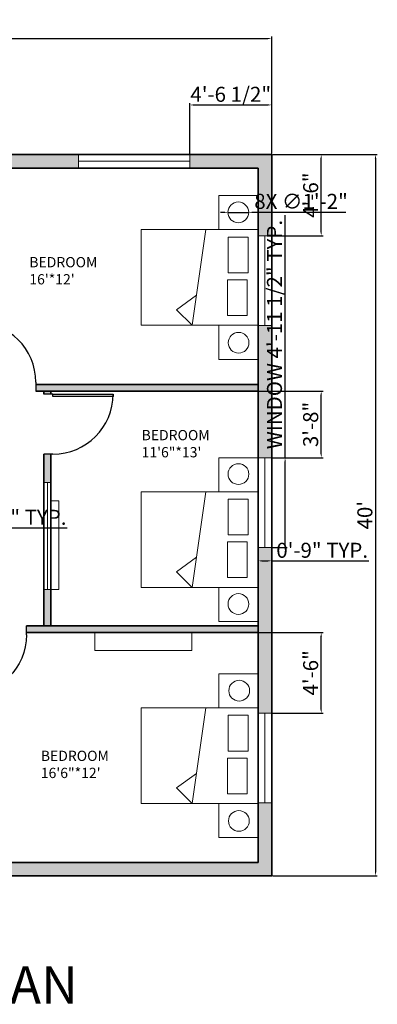
# Model space of a CAD drawing. Units: inches. Extents: x 1433 to 2137, y 2961 to 3626.
# Tile 3 of 3: x 1899 to 2137, y 2961 to 3616. Entities that reach past the tile are written whole.
import ezdxf

# ---------------------------------------------------------------- set-up
doc = ezdxf.new("R2010")
doc.units = ezdxf.units.IN
for name, color, linetype, lineweight in [('A-ANNO-DIMS', 2, 'Continuous', 18), ('A-ANNO-TEXT', 7, 'Continuous', 25), ('A-AREA-IDEN', 7, 'Continuous', 18), ('A-FURN', 8, 'Continuous', 18), ('A-WALL-PATT', 46, 'Continuous', 13), ('bed', 10, 'Continuous', 18), ('door', 50, 'Continuous', 25), ('wall', 46, 'Continuous', 35), ('window', 30, 'Continuous', 18)]:
    doc.layers.add(name, color=color, linetype=linetype, lineweight=lineweight)
doc.styles.get("Standard").update_dxf_attribs({"font": 'arial.ttf'})
doc.dimstyles.new('ISO-25', dxfattribs={"dimtxt": 10, "dimasz": 2.5, "dimexe": 1.25, "dimexo": 0.625, "dimtad": 1, "dimdec": 0, "dimlunit": 4, "dimtxsty": 'Standard', "dimcen": 2.5, "dimadec": 0, "dimazin": 0, "dimtfac": 1, "dimtdec": 0, "dimtmove": 0, "dimatfit": 3, "dimfxl": 1, "dimarcsym": 0})

# ---------------------------------------------------------------- blocks, each defined once
blk = doc.blocks.new('*U2')
for p, q in [((0, 0), (0, -6)), ((40, 0), (40, -6))]:
    blk.add_line(p, q)
blk.add_lwpolyline([(0, 0), (0, 40), (1.75, 40), (1.75, 0)], close=True)
blk.add_arc((0, 0), 40, 0, 90)
blk = doc.blocks.new('*D7')
at = {"layer": 'A-ANNO-DIMS', "color": 0, "lineweight": -2, "transparency": 16777216}
for p, q in [((1486.74, 3526.92), (1486.74, 3604.69)), ((1489.24, 3603.44), (2064.24, 3603.44)), ((2066.74, 3526.92), (2066.74, 3604.69))]:
    blk.add_line(p, q, dxfattribs=at)
at = {"layer": 'A-ANNO-DIMS', "color": 0, "transparency": 16777216}
for points in [[(1489.24, 3603.85), (1489.24, 3603.02), (1486.74, 3603.44)], [(2064.24, 3603.85), (2064.24, 3603.02), (2066.74, 3603.44)]]:
    blk.add_solid(points, dxfattribs=at)
at = {"layer": 'Defpoints', "color": 0, "transparency": 16777216}
for p in [(2066.74, 3603.44), (1486.74, 3526.3), (2066.74, 3526.3)]:
    blk.add_point(p, dxfattribs=at)
at = {"layer": 'A-ANNO-DIMS', "color": 0, "transparency": 16777216, "insert": (1776.74, 3609.17), "char_height": 10, "attachment_point": 5}
blk.add_mtext('48\'-4"', dxfattribs=at)
blk = doc.blocks.new('*D8')
at = {"layer": 'A-ANNO-DIMS', "color": 0, "lineweight": -2, "transparency": 16777216}
for p, q in [((2067.36, 3526.3), (2137.01, 3526.3)), ((2135.76, 3523.8), (2135.76, 3048.8)), ((2067.36, 3046.3), (2137.01, 3046.3))]:
    blk.add_line(p, q, dxfattribs=at)
at = {"layer": 'A-ANNO-DIMS', "color": 0, "transparency": 16777216}
for points in [[(2135.35, 3523.8), (2136.18, 3523.8), (2135.76, 3526.3)], [(2135.35, 3048.8), (2136.18, 3048.8), (2135.76, 3046.3)]]:
    blk.add_solid(points, dxfattribs=at)
at = {"layer": 'Defpoints', "color": 0, "transparency": 16777216}
for p in [(2066.74, 3526.3), (2066.74, 3046.3), (2135.76, 3046.3)]:
    blk.add_point(p, dxfattribs=at)
at = {"layer": 'A-ANNO-DIMS', "color": 0, "transparency": 16777216, "insert": (2130.03, 3286.3), "char_height": 10, "attachment_point": 5, "rotation": 90}
blk.add_mtext("40'", dxfattribs=at)
blk = doc.blocks.new('BED-DOUBLE-SIDE-TABLES')
for p, q in [((34.88, 22.67), (43.9, 86.32)), ((43.9, 86.32), (54.29, 75.94)), ((54.29, 75.94), (41.05, 66.2))]:
    blk.add_line(p, q)
for points in [[(0, 86.32), (26.13, 86.32), (26.13, 108.99), (0, 108.99)], [(0, 22.67), (77.8, 22.67), (77.8, 86.32), (0, 86.32)], [(7.27, 56), (20.39, 56), (20.39, 79.76), (7.27, 79.76)], [(6.72, 27.59), (19.84, 27.59), (19.84, 51.35), (6.72, 51.35)], [(0, 0), (26.13, 0), (26.13, 22.67), (0, 22.67)]]:
    blk.add_lwpolyline(points, close=True)
blk = doc.blocks.new('WIN-EXTERIOR-59_67IN')
blk.add_line((4.5, 0), (4.5, 59.67))
blk.add_lwpolyline([(0, 59.67), (9, 59.67), (9, 0), (0, 0)], close=True)
blk = doc.blocks.new('WIN-EXTERIOR-74_12IN')
blk.add_line((0, 4.5), (74.12, 4.5))
blk.add_lwpolyline([(0, 9), (74.12, 9), (74.12, 0), (0, 0)], close=True)
blk = doc.blocks.new('*D16')
at = {"layer": 'A-ANNO-DIMS', "color": 0, "lineweight": -2, "transparency": 16777216}
for p, q in [((2075.69, 3324.56), (2075.69, 3485.92)), ((2067.36, 3324.56), (2076.94, 3324.56)), ((2075.69, 3267.39), (2075.69, 3322.06)), ((2067.36, 3264.89), (2076.94, 3264.89))]:
    blk.add_line(p, q, dxfattribs=at)
at = {"layer": 'A-ANNO-DIMS', "color": 0, "transparency": 16777216}
for points in [[(2075.27, 3322.06), (2076.11, 3322.06), (2075.69, 3324.56)], [(2075.27, 3267.39), (2076.11, 3267.39), (2075.69, 3264.89)]]:
    blk.add_solid(points, dxfattribs=at)
at = {"layer": 'Defpoints', "color": 0, "transparency": 16777216}
for p in [(2066.74, 3324.56), (2075.69, 3324.56), (2066.74, 3264.89)]:
    blk.add_point(p, dxfattribs=at)
at = {"layer": 'A-ANNO-DIMS', "color": 0, "transparency": 16777216, "insert": (2069.89, 3406.49), "char_height": 10, "attachment_point": 5, "rotation": 90}
blk.add_mtext('WINDOW 4\'-11 1/2" TYP.', dxfattribs=at)
blk = doc.blocks.new('*D17')
at = {"layer": 'A-ANNO-DIMS', "color": 0, "lineweight": -2, "transparency": 16777216}
for p, q in [((2057.74, 3264.26), (2057.74, 3254.69)), ((2066.74, 3264.26), (2066.74, 3254.69)), ((2060.24, 3255.94), (2064.24, 3255.94)), ((2066.74, 3255.94), (2131.44, 3255.94))]:
    blk.add_line(p, q, dxfattribs=at)
at = {"layer": 'A-ANNO-DIMS', "color": 0, "transparency": 16777216}
for points in [[(2060.24, 3256.35), (2060.24, 3255.52), (2057.74, 3255.94)], [(2064.24, 3256.35), (2064.24, 3255.52), (2066.74, 3255.94)]]:
    blk.add_solid(points, dxfattribs=at)
at = {"layer": 'Defpoints', "color": 0, "transparency": 16777216}
for p in [(2057.74, 3264.89), (2066.74, 3264.89), (2066.74, 3255.94)]:
    blk.add_point(p, dxfattribs=at)
at = {"layer": 'A-ANNO-DIMS', "color": 0, "transparency": 16777216, "insert": (2100.34, 3261.67), "char_height": 10, "attachment_point": 5}
blk.add_mtext('0\'-9" TYP.', dxfattribs=at)
blk = doc.blocks.new('*D23')
at = {"layer": 'A-ANNO-DIMS', "color": 0, "lineweight": -2, "transparency": 16777216}
for p, q in [((1814.22, 3281.79), (1814.22, 3276.56)), ((1816.72, 3277.81), (1840.1, 3277.81)), ((1842.6, 3281.79), (1842.6, 3276.56)), ((1842.6, 3277.81), (1930.78, 3277.81))]:
    blk.add_line(p, q, dxfattribs=at)
at = {"layer": 'A-ANNO-DIMS', "color": 0, "transparency": 16777216}
for points in [[(1816.72, 3278.23), (1816.72, 3277.39), (1814.22, 3277.81)], [(1840.1, 3278.23), (1840.1, 3277.39), (1842.6, 3277.81)]]:
    blk.add_solid(points, dxfattribs=at)
at = {"layer": 'Defpoints', "color": 0, "transparency": 16777216}
for p in [(1814.22, 3282.42), (1842.6, 3282.42), (1842.6, 3277.81)]:
    blk.add_point(p, dxfattribs=at)
at = {"layer": 'A-ANNO-DIMS', "color": 0, "transparency": 16777216, "insert": (1887.94, 3283.61), "char_height": 10, "attachment_point": 5}
blk.add_mtext('2\'-4 1/2" TYP.', dxfattribs=at)
blk = doc.blocks.new('*D28')
at = {"layer": 'A-ANNO-DIMS', "color": 0, "lineweight": -2, "transparency": 16777216}
for p, q in [((2012.26, 3526.92), (2012.26, 3560.5)), ((2014.76, 3559.25), (2064.24, 3559.25)), ((2066.74, 3526.92), (2066.74, 3560.5))]:
    blk.add_line(p, q, dxfattribs=at)
at = {"layer": 'A-ANNO-DIMS', "color": 0, "transparency": 16777216}
for points in [[(2014.76, 3559.66), (2014.76, 3558.83), (2012.26, 3559.25)], [(2064.24, 3559.66), (2064.24, 3558.83), (2066.74, 3559.25)]]:
    blk.add_solid(points, dxfattribs=at)
at = {"layer": 'Defpoints', "color": 0, "transparency": 16777216}
for p in [(2066.74, 3559.25), (2012.26, 3526.3), (2066.74, 3526.3)]:
    blk.add_point(p, dxfattribs=at)
at = {"layer": 'A-ANNO-DIMS', "color": 0, "transparency": 16777216, "insert": (2039.5, 3565.04), "char_height": 10, "attachment_point": 5}
blk.add_mtext('4\'-6 1/2"', dxfattribs=at)
blk = doc.blocks.new('*D29')
at = {"layer": 'A-ANNO-DIMS', "color": 0, "lineweight": -2, "transparency": 16777216}
for p, q in [((2067.36, 3526.3), (2100.94, 3526.3)), ((2099.69, 3474.69), (2099.69, 3523.8)), ((2067.36, 3472.19), (2100.94, 3472.19))]:
    blk.add_line(p, q, dxfattribs=at)
at = {"layer": 'A-ANNO-DIMS', "color": 0, "transparency": 16777216}
for points in [[(2099.27, 3523.8), (2100.11, 3523.8), (2099.69, 3526.3)], [(2099.27, 3474.69), (2100.11, 3474.69), (2099.69, 3472.19)]]:
    blk.add_solid(points, dxfattribs=at)
at = {"layer": 'Defpoints', "color": 0, "transparency": 16777216}
for p in [(2066.74, 3526.3), (2099.69, 3526.3), (2066.74, 3472.19)]:
    blk.add_point(p, dxfattribs=at)
at = {"layer": 'A-ANNO-DIMS', "color": 0, "transparency": 16777216, "insert": (2093.96, 3499.24), "char_height": 10, "attachment_point": 5, "rotation": 90}
blk.add_mtext('4\'-6"', dxfattribs=at)
blk = doc.blocks.new('*D30')
at = {"layer": 'A-ANNO-DIMS', "color": 0, "lineweight": -2, "transparency": 16777216}
for p, q in [((2058.36, 3208.3), (2100.94, 3208.3)), ((2099.69, 3157.03), (2099.69, 3205.8)), ((2067.36, 3154.53), (2100.94, 3154.53))]:
    blk.add_line(p, q, dxfattribs=at)
at = {"layer": 'A-ANNO-DIMS', "color": 0, "transparency": 16777216}
for points in [[(2099.27, 3205.8), (2100.11, 3205.8), (2099.69, 3208.3)], [(2099.27, 3157.03), (2100.11, 3157.03), (2099.69, 3154.53)]]:
    blk.add_solid(points, dxfattribs=at)
at = {"layer": 'Defpoints', "color": 0, "transparency": 16777216}
for p in [(2057.74, 3208.3), (2099.69, 3208.3), (2066.74, 3154.53)]:
    blk.add_point(p, dxfattribs=at)
at = {"layer": 'A-ANNO-DIMS', "color": 0, "transparency": 16777216, "insert": (2093.96, 3181.41), "char_height": 10, "attachment_point": 5, "rotation": 90}
blk.add_mtext('4\'-6"', dxfattribs=at)
blk = doc.blocks.new('*D31')
at = {"layer": 'A-ANNO-DIMS', "color": 0, "lineweight": -2, "transparency": 16777216}
for p, q in [((2058.36, 3368.8), (2100.94, 3368.8)), ((2099.69, 3327.06), (2099.69, 3366.3)), ((2067.36, 3324.56), (2100.94, 3324.56))]:
    blk.add_line(p, q, dxfattribs=at)
at = {"layer": 'A-ANNO-DIMS', "color": 0, "transparency": 16777216}
for points in [[(2099.27, 3366.3), (2100.11, 3366.3), (2099.69, 3368.8)], [(2099.27, 3327.06), (2100.11, 3327.06), (2099.69, 3324.56)]]:
    blk.add_solid(points, dxfattribs=at)
at = {"layer": 'Defpoints', "color": 0, "transparency": 16777216}
for p in [(2057.74, 3368.8), (2099.69, 3368.8), (2066.74, 3324.56)]:
    blk.add_point(p, dxfattribs=at)
at = {"layer": 'A-ANNO-DIMS', "color": 0, "transparency": 16777216, "insert": (2093.96, 3346.68), "char_height": 10, "attachment_point": 5, "rotation": 90}
blk.add_mtext('3\'-8"', dxfattribs=at)
blk = doc.blocks.new('*D39')
at = {"layer": 'A-ANNO-DIMS', "color": 0, "lineweight": -2, "transparency": 16777216}
for p, q in [((2035.13, 3487.81), (2032.63, 3487.81)), ((2037.63, 3487.81), (2051.43, 3487.81)), ((2116.11, 3487.81), (2053.93, 3487.81))]:
    blk.add_line(p, q, dxfattribs=at)
at = {"layer": 'A-ANNO-DIMS', "color": 0, "transparency": 16777216}
for points in [[(2035.13, 3488.23), (2035.13, 3487.39), (2037.63, 3487.81)], [(2053.93, 3488.23), (2053.93, 3487.39), (2051.43, 3487.81)]]:
    blk.add_solid(points, dxfattribs=at)
at = {"layer": 'Defpoints', "color": 0, "transparency": 16777216}
for p in [(2037.63, 3487.81), (2051.43, 3487.81)]:
    blk.add_point(p, dxfattribs=at)
at = {"layer": 'A-ANNO-DIMS', "color": 0, "transparency": 16777216, "insert": (2086.27, 3493.82), "char_height": 10, "attachment_point": 5, "rotation": 0.0015}
blk.add_mtext('8X ∅1\'-2"', dxfattribs=at)

msp = doc.modelspace()

# ---------------------------------------------------------------- hatches: boundary and pattern name
at = {"layer": 'A-WALL-PATT'}
h = msp.add_hatch(color=256, dxfattribs=at)
h.dxf.hatch_style = 1
h.paths.add_polyline_path([(1542.09, 3526.3), (1486.74, 3526.3), (1486.74, 3471.83), (1495.74, 3471.83), (1495.74, 3475.8), (1495.74, 3517.3), (1542.09, 3517.3)])
h.paths.add_polyline_path([(2066.74, 3526.3), (2012.26, 3526.3), (2012.26, 3517.3), (2057.74, 3517.3), (2057.74, 3472.19), (2066.74, 3472.19)])
h.paths.add_polyline_path([(2066.74, 3412.52), (2057.74, 3412.52), (2057.74, 3389.96), (2057.74, 3324.56), (2066.74, 3324.56)])
h.paths.add_polyline_path([(2066.74, 3264.89), (2057.74, 3264.89), (2057.74, 3238.24), (2057.74, 3215.57), (2057.74, 3212.8), (2057.74, 3154.53), (2066.74, 3154.53)])
h = msp.add_hatch(color=256, dxfattribs=at)
h.dxf.hatch_style = 1
h.paths.add_polyline_path([(1684.74, 3526.3), (1616.21, 3526.3), (1616.21, 3517.3), (1684.74, 3517.3)])
h.paths.add_polyline_path([(1938.14, 3526.3), (1861.24, 3526.3), (1861.24, 3517.3), (1938.14, 3517.3)])
h = msp.add_hatch(color=256, dxfattribs=at)
h.dxf.hatch_style = 1
h.paths.add_polyline_path([(1684.74, 3517.3), (1675.74, 3517.3), (1675.74, 3405.93), (1679.92, 3405.93, -0.043454), (1684.74, 3405.51)])
h.paths.add_polyline_path([(1861.24, 3373.3), (1801.24, 3373.3), (1801.24, 3439.3), (1861.24, 3439.3), (1861.24, 3443.8), (1796.74, 3443.8), (1796.74, 3368.8), (1861.24, 3368.8)])
h.paths.add_polyline_path([(1749.24, 3443.8), (1684.74, 3443.8), (1684.74, 3439.3), (1744.74, 3439.3), (1744.74, 3373.3), (1684.74, 3373.3), (1684.74, 3368.8), (1749.24, 3368.8)])
h.paths.add_polyline_path([(1684.74, 3378.05), (1679.92, 3378.05), (1675.74, 3378.05), (1675.74, 3373.3), (1672.64, 3373.3), (1672.64, 3368.8), (1684.74, 3368.8), (1684.74, 3373.3)])
h.paths.add_polyline_path([(1865.74, 3378.26), (1861.56, 3378.26), (1861.24, 3378.26), (1861.24, 3368.8), (1869.81, 3368.8), (1869.81, 3373.3), (1865.74, 3373.3)])
h.paths.add_polyline_path([(2057.74, 3373.3), (1909.81, 3373.3), (1909.81, 3368.8), (2057.74, 3368.8)])
h.paths.add_polyline_path([(1919.74, 3368.8), (1915.24, 3368.8), (1915.24, 3366.92), (1919.74, 3366.92)])
h.paths.add_polyline_path([(1919.74, 3326.92), (1915.24, 3326.92), (1915.24, 3308.14), (1919.74, 3308.14)])
h.paths.add_polyline_path([(1919.74, 3236.84), (1915.24, 3236.84), (1915.24, 3212.8), (1919.74, 3212.8)])
h.paths.add_polyline_path([(1859.74, 3208.3), (1855.24, 3208.3), (1855.24, 3203.85), (1855.29, 3203.85), (1859.74, 3203.85)])
h = msp.add_hatch(color=256, dxfattribs=at)
h.dxf.hatch_style = 1
h.paths.add_polyline_path([(1632.64, 3373.3), (1495.74, 3373.3), (1495.74, 3368.8), (1632.64, 3368.8)])
h.paths.add_polyline_path([(1620.24, 3368.8), (1615.74, 3368.8), (1615.74, 3362.47), (1620.24, 3362.47)])
h.paths.add_polyline_path([(1526.85, 3272.8), (1495.74, 3272.8), (1495.74, 3268.3), (1526.85, 3268.3)])
h.paths.add_polyline_path([(1612.35, 3272.8), (1579.17, 3272.8), (1579.17, 3268.3), (1607.43, 3268.3), (1608.56, 3269.33)])
h.paths.add_polyline_path([(1620.24, 3275.2), (1620.24, 3280), (1608.56, 3269.33), (1607.43, 3268.3), (1613.07, 3268.3)])
h.paths.add_polyline_path([(1620.24, 3322.47), (1615.74, 3322.47), (1615.74, 3275.89), (1620.24, 3280)])
h.paths.add_polyline_path([(1621.12, 3270.32), (1618.48, 3273.5), (1615.2, 3270.34), (1617.74, 3267.34)])
h.paths.add_polyline_path([(1658.27, 3208.55), (1655.63, 3211.74), (1652.35, 3208.58), (1654.95, 3205.51)])
h.paths.add_polyline_path([(1564.19, 3050.13), (1564.19, 3055.3), (1540.78, 3055.3), (1540.78, 3049.3, -0.01877), (1540.67, 3046.3), (1564.19, 3046.3)])
h.paths.add_polyline_path([(1693.15, 3055.3), (1655.74, 3055.3), (1633.11, 3055.3), (1633.11, 3050.13), (1633.11, 3046.3), (1693.15, 3046.3)])
h.paths.add_polyline_path([(1804.24, 3127.3), (1804.24, 3208.3), (1799.74, 3208.3), (1799.74, 3131.8), (1799.74, 3055.3), (1804.24, 3055.3)])
h.paths.add_polyline_path([(1655.74, 3142.86), (1651.24, 3142.86), (1651.24, 3055.3), (1655.74, 3055.3)])
h.paths.add_polyline_path([(2057.74, 3212.8), (1903.59, 3212.8), (1903.59, 3208.3), (2057.74, 3208.3)])
h.paths.add_polyline_path([(1855.24, 3055.3), (1855.24, 3046.3), (2066.74, 3046.3), (2066.74, 3094.86), (2057.74, 3094.86), (2057.74, 3094.45), (2057.74, 3071.77), (2057.74, 3055.3)])

# ---------------------------------------------------------------- linework, layer by layer
at = {"layer": 'A-FURN'}
for points in [[(1919.74, 3236.84), (1925.07, 3236.84), (1925.07, 3295.87), (1919.74, 3295.87)], [(2013.59, 3208.3), (1949.06, 3208.3), (1949.06, 3196.23), (2013.59, 3196.23)]]:
    msp.add_lwpolyline(points, close=True, dxfattribs=at)
at = {"layer": 'bed'}
for centre in [(2044.53, 3487.81), (2044.74, 3401.04), (2044.63, 3313.67), (2044.61, 3227.22), (2045.13, 3169.56), (2044.92, 3082.88)]:
    msp.add_circle(centre, 6.9, dxfattribs=at)
at = {"layer": 'wall'}
for p, q in [((1790.89, 3526.3), (2066.74, 3526.3)), ((2066.74, 3526.3), (2066.74, 3046.3)), ((1861.24, 3517.3), (2057.74, 3517.3)), ((2057.74, 3517.3), (1865.74, 3517.3)), ((2057.74, 3517.3), (2057.74, 3055.3)), ((1909.81, 3373.3), (2057.74, 3373.3)), ((1909.81, 3368.8), (2057.74, 3368.8)), ((1915.24, 3366.92), (1915.24, 3368.8)), ((1919.74, 3366.92), (1919.74, 3368.8)), ((2057.74, 3368.8), (2057.74, 3212.8)), ((1915.24, 3212.8), (1915.24, 3326.92)), ((1919.74, 3212.8), (1919.74, 3326.92)), ((2057.74, 3212.8), (1903.59, 3212.8)), ((2057.74, 3212.8), (1919.74, 3212.8)), ((2057.74, 3208.3), (1903.59, 3208.3)), ((2057.74, 3208.3), (1915.24, 3208.3)), ((2057.74, 3055.3), (1855.24, 3055.3)), ((2066.74, 3046.3), (1631.6, 3046.3))]:
    msp.add_line(p, q, dxfattribs=at)
at = {"layer": 'window'}
for p, q in [((1919.74, 3308.14), (1917.49, 3308.14)), ((1917.49, 3308.14), (1917.49, 3236.84))]:
    msp.add_line(p, q, dxfattribs=at)
msp.add_lwpolyline([(1915.24, 3308.14), (1919.74, 3308.14), (1919.74, 3236.84), (1915.24, 3236.84)], close=True, dxfattribs=at)

# ---------------------------------------------------------------- block references
at = {"layer": 'bed', "rotation": 180}
for p in [(2057.74, 3498.95), (2057.74, 3324.56), (2057.74, 3180.76)]:
    msp.add_blockref('BED-DOUBLE-SIDE-TABLES', p, dxfattribs=at)
at = {"layer": 'door'}
msp.add_blockref('*U2', (1869.81, 3374.8), dxfattribs=at)
at = {"layer": 'door', "rotation": 270}
msp.add_blockref('*U2', (1921.24, 3366.92), dxfattribs=at)
at = {"layer": 'door', "xscale": -1, "rotation": 180}
msp.add_blockref('*U2', (1863.59, 3206.8), dxfattribs=at)
at = {"layer": 'window'}
for name, p in [('WIN-EXTERIOR-74_12IN', (1938.14, 3517.3)), ('WIN-EXTERIOR-59_67IN', (2057.74, 3412.52)), ('WIN-EXTERIOR-59_67IN', (2057.74, 3264.89)), ('WIN-EXTERIOR-59_67IN', (2057.74, 3094.86))]:
    msp.add_blockref(name, p, dxfattribs=at)

# ---------------------------------------------------------------- texts
at = {"layer": 'A-ANNO-TEXT', "insert": (1634.97, 2986.23), "char_height": 24.8992, "attachment_point": 1}
msp.add_mtext_dynamic_manual_height_columns('4BHK HOUSE PLAN', width=495.0792, gutter_width=124.5, heights=[0], dxfattribs=at)
at = {"layer": 'A-AREA-IDEN', "char_height": 6.823, "attachment_point": 1}
for s, insert in [("BEDROOM\\P16'*12'", (1905.49, 3458.06)), ('BEDROOM\\P11\'6"*13\'', (1980.21, 3342.99)), ('BEDROOM\\P16\'6"*12\'', (1913.14, 3129.61))]:
    msp.add_mtext_dynamic_manual_height_columns(s, width=135.668, gutter_width=34.12, heights=[0], dxfattribs=dict(at, insert=insert))

# ---------------------------------------------------------------- dimensions: what is measured, and where the dimension line sits
at = {"layer": 'A-ANNO-DIMS'}
for base, p1, override, picture, middle in [((2066.74, 3603.44), (1486.74, 3526.3), {"dimclrd": 0, "dimclre": 0, "dimclrt": 0}, '*D7', (1776.74, 3609.17)), ((2066.74, 3559.25), (2012.26, 3526.3), {"dimdec": 1, "dimlfac": 1, "dimrnd": 0, "dimzin": 1, "dimdsep": 46, "dimlunit": 4, "dimfrac": 2}, '*D28', (2039.5, 3565.04))]:
    dim = msp.add_linear_dim(base=base, p1=p1, p2=(2066.74, 3526.3), dimstyle='ISO-25', override=override, dxfattribs=at)
    dim.commit()
    dim.dimension.update_dxf_attribs({"geometry": picture, "text_midpoint": middle})
for base, p1, p2, override, picture, middle in [((2135.76, 3046.3), (2066.74, 3526.3), (2066.74, 3046.3), {"dimclrd": 0, "dimclre": 0, "dimclrt": 0}, '*D8', (2130.03, 3286.3)), ((2099.69, 3526.3), (2066.74, 3472.19), (2066.74, 3526.3), {"dimdec": 1, "dimlfac": 1, "dimrnd": 0, "dimzin": 1, "dimdsep": 46, "dimlunit": 4, "dimfrac": 2}, '*D29', (2093.96, 3499.24)), ((2099.69, 3368.8), (2066.74, 3324.56), (2057.74, 3368.8), {"dimdec": 1, "dimlfac": 1, "dimrnd": 0, "dimzin": 1, "dimdsep": 46, "dimlunit": 4, "dimfrac": 2}, '*D31', (2093.96, 3346.68)), ((2099.69, 3208.3), (2066.74, 3154.53), (2057.74, 3208.3), {"dimdec": 1, "dimlfac": 1, "dimrnd": 0, "dimzin": 1, "dimdsep": 46, "dimlunit": 4, "dimfrac": 2}, '*D30', (2093.96, 3181.41))]:
    dim = msp.add_linear_dim(base=base, p1=p1, p2=p2, angle=90, dimstyle='ISO-25', override=override, dxfattribs=at)
    dim.commit()
    dim.dimension.update_dxf_attribs({"geometry": picture, "text_midpoint": middle})
dim = msp.add_diameter_dim_2p(p1=(2037.63, 3487.81), p2=(2051.43, 3487.81), text='8X <>', dimstyle='ISO-25', override={"dimdec": 1, "dimlfac": 1, "dimrnd": 0, "dimzin": 1, "dimdsep": 46, "dimlunit": 4, "dimfrac": 2}, dxfattribs=at)
dim.commit()
dim.dimension.update_dxf_attribs({"geometry": '*D39', "text_midpoint": (2086.27, 3487.81), "dimtype": 163})
dim = msp.add_linear_dim(base=(2075.69, 3324.56), p1=(2066.74, 3264.89), p2=(2066.74, 3324.56), angle=90, text='WINDOW <> TYP.', dimstyle='ISO-25', override={"dimdec": 1, "dimlfac": 1, "dimrnd": 0, "dimzin": 1, "dimdsep": 46, "dimlunit": 4, "dimfrac": 2}, dxfattribs=at)
dim.commit()
dim.dimension.update_dxf_attribs({"geometry": '*D16', "text_midpoint": (2069.89, 3406.49)})
for base, p1, p2, picture, middle in [((1842.6, 3277.81), (1814.22, 3282.42), (1842.6, 3282.42), '*D23', (1887.94, 3283.61)), ((2066.74, 3255.94), (2057.74, 3264.89), (2066.74, 3264.89), '*D17', (2100.34, 3261.67))]:
    dim = msp.add_linear_dim(base=base, p1=p1, p2=p2, text='<> TYP.', dimstyle='ISO-25', override={"dimdec": 1, "dimlfac": 1, "dimrnd": 0, "dimzin": 1, "dimdsep": 46, "dimlunit": 4, "dimfrac": 2}, dxfattribs=at)
    dim.commit()
    dim.dimension.update_dxf_attribs({"geometry": picture, "text_midpoint": middle})

doc.saveas('drawing.dxf')
